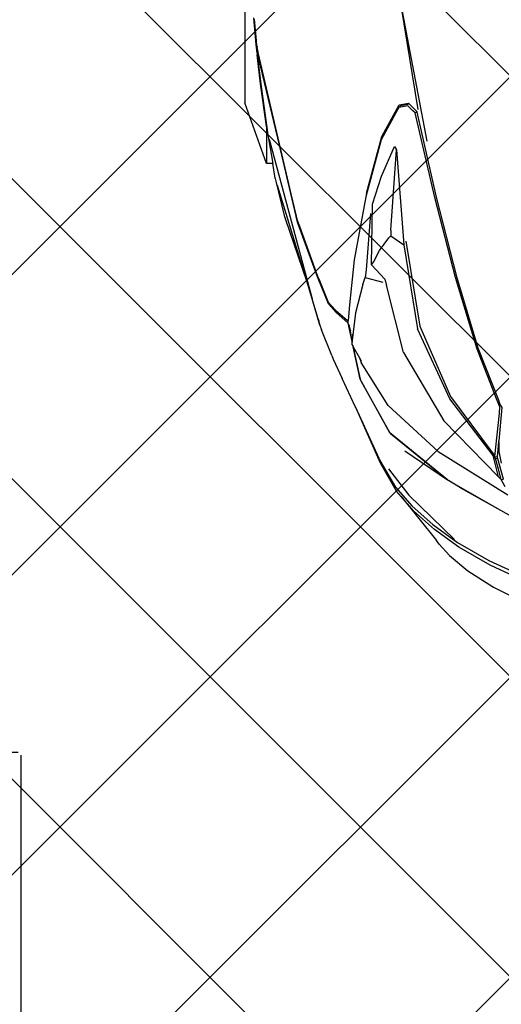
# Model space of a CAD drawing. Units: inches. Extents: x 2167 to 2589, y 1680 to 2489.
# Tile 3 of 38: x 2251.19 to 2262.53, y 1703.49 to 1726.68. Entities that reach past the tile are written whole.
import ezdxf

# ---------------------------------------------------------------- set-up
doc = ezdxf.new("R2010")
doc.units = ezdxf.units.IN
doc.header["$MEASUREMENT"] = 0
doc.layers.get('0').update_dxf_attribs({"color": 250})
for name, color, linetype, lineweight in [('A-ANNO-DIMS', 2, 'Continuous', 18), ('C-PRKG-VEHS', 8, 'Continuous', 13), ('L-PVMT-PATT', 252, 'Continuous', 13)]:
    doc.layers.add(name, color=color, linetype=linetype, lineweight=lineweight)
doc.layers.add('Edges', color=250, linetype='Continuous')
doc.styles.get("Standard").update_dxf_attribs({"font": 'arial.ttf'})
doc.dimstyles.get("Standard").update_dxf_attribs({"dimtxt": 7, "dimasz": 0.18, "dimexe": 0.18, "dimexo": 0.0625, "dimgap": 0.09, "dimtad": 0, "dimtih": 1, "dimtoh": 1, "dimdec": 1, "dimzin": 0, "dimdsep": 46, "dimlunit": 3, "dimtxsty": 'Standard', "dimcen": 0.09, "dimadec": 0, "dimazin": 0, "dimtfac": 1, "dimtdec": 1, "dimtofl": 0, "dimtmove": 0, "dimatfit": 3, "dimfxl": 1, "dimtolj": 1, "dimtzin": 0, "dimarcsym": 0})

# ---------------------------------------------------------------- blocks, each defined once
blk = doc.blocks.new('Nissan Qashqai pl')
at = {"layer": 'Edges'}
for p, q in [((11.47322, 11.2592), (11.46579, 11.24614)), ((11.50736, 11.23616), (11.51652, 11.25601)), ((11.52058, 11.25724), (11.51126, 11.23721)), ((11.52949, 11.24004), (11.53843, 11.2583)), ((11.41698, 11.19425), (11.45295, 11.25195)), ((11.43996, 11.24823), (11.42296, 11.24352)), ((11.44027, 11.24637), (11.43996, 11.24823)), ((11.44624, 11.24948), (11.44027, 11.24637)), ((11.33108, 11.22699), (11.37506, 11.24429)), ((11.37475, 11.24309), (11.33228, 11.22637)), ((11.42033, 11.23975), (11.37334, 11.20375)), ((11.38, 11.24532), (11.37475, 11.24309)), ((11.37506, 11.24429), (11.37524, 11.24436)), ((11.37506, 11.24429), (11.37621, 11.24429)), ((11.37922, 11.24593), (11.37524, 11.24436)), ((11.3763, 11.24436), (11.37524, 11.24436)), ((11.37922, 11.24593), (11.38041, 11.24692)), ((11.37933, 11.24631), (11.37922, 11.24593)), ((11.38533, 11.24487), (11.38, 11.24532)), ((11.38041, 11.24692), (11.40818, 11.24436)), ((11.42115, 11.24117), (11.38533, 11.24487)), ((11.3915, 11.19885), (11.4381, 11.24397)), ((11.41644, 11.24436), (11.40818, 11.24436)), ((11.40898, 11.24429), (11.40818, 11.24436)), ((11.40898, 11.24429), (11.4163, 11.24429)), ((11.4152, 11.24371), (11.40898, 11.24429)), ((11.4163, 11.24429), (11.4152, 11.24371)), ((11.42154, 11.24313), (11.4152, 11.24371)), ((11.41644, 11.24436), (11.4163, 11.24429)), ((11.41686, 11.24458), (11.41644, 11.24436)), ((11.4252, 11.2462), (11.41686, 11.24458)), ((11.41772, 11.23895), (11.41931, 11.23998)), ((11.41915, 11.23969), (11.4194, 11.23996)), ((11.41931, 11.23998), (11.4196, 11.24017)), ((11.4194, 11.23996), (11.41931, 11.23998)), ((11.4194, 11.23996), (11.4196, 11.24017)), ((11.41958, 11.23992), (11.4194, 11.23996)), ((11.4196, 11.24017), (11.42014, 11.24052)), ((11.41984, 11.24006), (11.42014, 11.24052)), ((11.42014, 11.24052), (11.42115, 11.24117)), ((11.42915, 11.24177), (11.42033, 11.23975)), ((11.42287, 11.24164), (11.42033, 11.23975)), ((11.42115, 11.24117), (11.42154, 11.24313)), ((11.42178, 11.24134), (11.42115, 11.24117)), ((11.42296, 11.24352), (11.42154, 11.24313)), ((11.42287, 11.24164), (11.42178, 11.24134)), ((11.42216, 11.24127), (11.42178, 11.24134)), ((11.43154, 11.24397), (11.42287, 11.24164)), ((11.42296, 11.24352), (11.42287, 11.24164)), ((11.42659, 11.2465), (11.4252, 11.2462)), ((11.4381, 11.24397), (11.42915, 11.24177)), ((11.44027, 11.24637), (11.43154, 11.24397)), ((11.4381, 11.24397), (11.44027, 11.24637)), ((11.44114, 11.20281), (11.46562, 11.24583)), ((11.44697, 11.21272), (11.46562, 11.24583)), ((11.46562, 11.24583), (11.46579, 11.24614)), ((11.51576, 11.21859), (11.52949, 11.24004)), ((11.3715, 11.20434), (11.41772, 11.23895)), ((11.49236, 11.21027), (11.50736, 11.23616)), ((11.51126, 11.23721), (11.49628, 11.21137)), ((11.27199, 11.20923), (11.33108, 11.22699)), ((11.33228, 11.22637), (11.27276, 11.20843)), ((11.50327, 11.20341), (11.51576, 11.21859)), ((11.20627, 11.19262), (11.27199, 11.20923)), ((11.27276, 11.20843), (11.20665, 11.19145)), ((11.44697, 11.21272), (11.44114, 11.20281)), ((11.45306, 11.16974), (11.48975, 11.20767)), ((11.47745, 11.18983), (11.49236, 11.21027)), ((11.49628, 11.21137), (11.48154, 11.19102)), ((11.31316, 11.17892), (11.3715, 11.20434)), ((11.37334, 11.20375), (11.31527, 11.17691)), ((11.33497, 11.16556), (11.3915, 11.19885)), ((11.44046, 11.20182), (11.40144, 11.15414)), ((11.40216, 11.15476), (11.44046, 11.20182)), ((11.41633, 11.16662), (11.44046, 11.20182)), ((11.44081, 11.20225), (11.44046, 11.20182)), ((11.4411, 11.20277), (11.44081, 11.20225)), ((11.44114, 11.20281), (11.4411, 11.20277)), ((11.50327, 11.20341), (11.49363, 11.19502)), ((11.20665, 11.19145), (11.14012, 11.17593)), ((11.14803, 11.17913), (11.20627, 11.19262)), ((11.37896, 11.15265), (11.41698, 11.19425)), ((11.45433, 11.16358), (11.49082, 11.19282)), ((11.48154, 11.19102), (11.46617, 11.17358)), ((11.49363, 11.19502), (11.49082, 11.19282)), ((11.03575, 11.16129), (11.1598, 11.18473)), ((11.46237, 11.17248), (11.47745, 11.18983)), ((11.04919, 11.16347), (11.13359, 11.17719)), ((11.12929, 11.17052), (11.13526, 11.17642)), ((11.13658, 11.17502), (11.1347, 11.17313)), ((11.13526, 11.17642), (11.13585, 11.17654)), ((11.13585, 11.17654), (11.14803, 11.17913)), ((11.13585, 11.17654), (11.13658, 11.17502)), ((11.14012, 11.17593), (11.13658, 11.17502)), ((11.24278, 11.16729), (11.31316, 11.17892)), ((11.24587, 11.16563), (11.31527, 11.17691)), ((11.12846, 11.16971), (11.12929, 11.17052)), ((11.12977, 11.16183), (11.12846, 11.16971)), ((11.12929, 11.17052), (11.13057, 11.16299)), ((11.1347, 11.17313), (11.13062, 11.16899)), ((11.13062, 11.16899), (11.13192, 11.16144)), ((11.43143, 11.15309), (11.45306, 11.16974)), ((11.44642, 11.15882), (11.46237, 11.17248)), ((11.46617, 11.17358), (11.45433, 11.16358)), ((11.15597, 11.14759), (11.12977, 11.16183)), ((11.13192, 11.16144), (11.13057, 11.16299)), ((11.13192, 11.16144), (11.13652, 11.15905)), ((11.13652, 11.15905), (11.15893, 11.14704)), ((11.16444, 11.15792), (11.16717, 11.15976)), ((11.18896, 11.14734), (11.16444, 11.15792)), ((11.16717, 11.15976), (11.24587, 11.16563)), ((11.23369, 11.15498), (11.16717, 11.15976)), ((11.23823, 11.15494), (11.24587, 11.16563)), ((11.33497, 11.16556), (11.27913, 11.15147)), ((11.42433, 11.14593), (11.44642, 11.15882)), ((11.44983, 11.15977), (11.42671, 11.14629)), ((11.45433, 11.16358), (11.44983, 11.15977)), ((11.23369, 11.15498), (11.23823, 11.15494)), ((11.23823, 11.15494), (11.2401, 11.15337)), ((11.25046, 11.1455), (11.2401, 11.15337)), ((11.27429, 11.14993), (11.26224, 11.13901)), ((11.27429, 11.14993), (11.27913, 11.15147)), ((11.37896, 11.15265), (11.34336, 11.13032)), ((11.40144, 11.15414), (11.3571, 11.12956)), ((11.35832, 11.12998), (11.40144, 11.15414)), ((11.40216, 11.15476), (11.40144, 11.15414)), ((11.20291, 11.13489), (11.15597, 11.14759)), ((11.15893, 11.14704), (11.20616, 11.13437)), ((11.2121, 11.1399), (11.18896, 11.14734)), ((11.26005, 11.1405), (11.25046, 11.1455)), ((11.27289, 11.13379), (11.27664, 11.14845)), ((11.42671, 11.14629), (11.38067, 11.12595)), ((11.42283, 11.14525), (11.38067, 11.12595)), ((11.42283, 11.14525), (11.42433, 11.14593)), ((11.20291, 11.13489), (11.20295, 11.13488)), ((11.20295, 11.13488), (11.20616, 11.13437)), ((11.20616, 11.13437), (11.25827, 11.12461)), ((11.26224, 11.13901), (11.2121, 11.1399)), ((11.21991, 11.1382), (11.26663, 11.13449)), ((11.26224, 11.13901), (11.26005, 11.1405)), ((11.26663, 11.13449), (11.27289, 11.13379)), ((11.27871, 11.13184), (11.27289, 11.13379)), ((11.27871, 11.13184), (11.30218, 11.1256)), ((11.30218, 11.1256), (11.32517, 11.12286)), ((11.32955, 11.12347), (11.3571, 11.12956)), ((11.3571, 11.12956), (11.33021, 11.12384)), ((11.33021, 11.12384), (11.33938, 11.12898)), ((11.33938, 11.12898), (11.34202, 11.13045)), ((11.33938, 11.12898), (11.34336, 11.13032)), ((11.37962, 11.12547), (11.35656, 11.11477)), ((11.3571, 11.12956), (11.35832, 11.12998)), ((11.38067, 11.12595), (11.37962, 11.12547)), ((11.25827, 11.12461), (11.29558, 11.12077)), ((11.29558, 11.12077), (11.30849, 11.1195)), ((11.30003, 11.10916), (11.30813, 11.11883)), ((11.31027, 11.11923), (11.30178, 11.10961)), ((11.30805, 11.11884), (11.30863, 11.11948)), ((11.30813, 11.11883), (11.30863, 11.11948)), ((11.30849, 11.1195), (11.30863, 11.11948)), ((11.30863, 11.11948), (11.31033, 11.1193)), ((11.31033, 11.1193), (11.31027, 11.11923)), ((11.31033, 11.1193), (11.31061, 11.11927)), ((11.31061, 11.11927), (11.314, 11.12039)), ((11.31704, 11.12142), (11.31186, 11.12058)), ((11.31323, 11.11986), (11.32588, 11.12266)), ((11.32423, 11.12258), (11.314, 11.12039)), ((11.314, 11.12039), (11.31704, 11.12142)), ((11.32423, 11.12258), (11.31704, 11.12142)), ((11.31982, 11.1231), (11.32517, 11.12286)), ((11.32423, 11.12258), (11.32588, 11.12266)), ((11.32517, 11.12286), (11.32831, 11.12278)), ((11.32588, 11.12266), (11.32831, 11.12278)), ((11.32831, 11.12278), (11.32955, 11.12347)), ((11.32955, 11.12347), (11.33021, 11.12384)), ((11.29339, 11.10313), (11.30003, 11.10916)), ((11.30178, 11.10961), (11.29459, 11.10327)), ((11.34052, 11.10725), (11.35656, 11.11477)), ((11.29459, 11.10327), (11.27358, 11.0947)), ((11.27407, 11.09522), (11.29339, 11.10313)), ((11.33757, 11.10603), (11.31612, 11.09747)), ((11.33757, 11.10603), (11.34052, 11.10725)), ((11.2732, 11.09452), (11.22772, 11.07792)), ((11.23038, 11.07923), (11.27187, 11.09432)), ((11.27187, 11.09432), (11.27407, 11.09522)), ((11.27358, 11.0947), (11.2732, 11.09452)), ((11.27358, 11.0947), (11.27407, 11.09522)), ((11.27568, 11.08503), (11.31244, 11.09628)), ((11.31244, 11.09628), (11.29065, 11.08989)), ((11.30801, 11.09508), (11.30877, 11.09528)), ((11.31244, 11.09628), (11.31612, 11.09747)), ((11.15816, 11.05423), (11.29065, 11.08989)), ((11.19633, 11.06072), (11.27568, 11.08503)), ((11.22475, 11.06772), (11.27568, 11.08503)), ((11.22216, 11.0766), (11.08821, 11.045)), ((11.09177, 11.04531), (11.22216, 11.0766)), ((11.21998, 11.07614), (11.22216, 11.0766)), ((11.2222, 11.07656), (11.22216, 11.0766)), ((11.22715, 11.07771), (11.2222, 11.07656)), ((11.22238, 11.07665), (11.2222, 11.07656)), ((11.22238, 11.07665), (11.22532, 11.07737)), ((11.22532, 11.07737), (11.23038, 11.07923)), ((11.22731, 11.07783), (11.22706, 11.07777)), ((11.22962, 11.07837), (11.22715, 11.07771)), ((11.22772, 11.07792), (11.22715, 11.07771)), ((11.22962, 11.07837), (11.22772, 11.07792)), ((11.08649, 11.04496), (11.21998, 11.07614)), ((11.19297, 11.05964), (11.22148, 11.06662)), ((11.22148, 11.06662), (11.22475, 11.06772)), ((11.14751, 11.05208), (11.11234, 11.04716)), ((11.11474, 11.04762), (11.15472, 11.05317)), ((11.17828, 11.05208), (11.12828, 11.03408)), ((11.15248, 11.05278), (11.14751, 11.05208)), ((11.14751, 11.05208), (11.17828, 11.05208)), ((11.15472, 11.05317), (11.15248, 11.05278)), ((11.15472, 11.05317), (11.17828, 11.05716)), ((11.19065, 11.05923), (11.17828, 11.05716)), ((11.17828, 11.05716), (11.17828, 11.05208)), ((11.19089, 11.05929), (11.19065, 11.05923)), ((11.19089, 11.05929), (11.19297, 11.05964)), ((11.07681, 11.04337), (11.08106, 11.04371)), ((11.08696, 11.04422), (11.07977, 11.04339)), ((11.08106, 11.04371), (11.08273, 11.0441)), ((11.08114, 11.04436), (11.08208, 11.0442)), ((11.08273, 11.0441), (11.08562, 11.04476)), ((11.08273, 11.0441), (11.08365, 11.04395)), ((11.08821, 11.045), (11.08365, 11.04395)), ((11.08365, 11.04395), (11.08696, 11.04422)), ((11.08562, 11.04476), (11.08649, 11.04496)), ((11.08649, 11.04496), (11.08796, 11.04514)), ((11.08696, 11.04422), (11.08721, 11.04424)), ((11.08728, 11.04426), (11.08721, 11.04424)), ((11.08728, 11.04426), (11.08834, 11.04438)), ((11.08834, 11.04438), (11.11474, 11.04762)), ((11.11234, 11.04716), (11.08834, 11.04438)), ((11.07977, 11.04339), (11.05762, 11.04159)), ((11.05899, 11.04188), (11.07681, 11.04337)), ((10.95773, 11.03408), (11.12828, 11.03408))]:
    blk.add_line(p, q, dxfattribs=at)
blk = doc.blocks.new('car')
blk.add_blockref('Nissan Qashqai pl', (-9.74328, -11.91512))
blk = doc.blocks.new('carr')
blk.add_blockref('car', (0.51244, -0.00696))
blk = doc.blocks.new('*D45')
at = {"layer": 'A-ANNO-DIMS', "color": 0, "lineweight": -2, "transparency": 16777216}
for p, q in [((2251.156, 1833.955), (2232.359, 1833.955)), ((2232.539, 1833.775), (2232.539, 1775.399)), ((2232.539, 1709.605), (2232.539, 1767.981)), ((2251.156, 1709.425), (2232.359, 1709.425))]:
    blk.add_line(p, q, dxfattribs=at)
at = {"layer": 'A-ANNO-DIMS', "color": 0, "transparency": 16777216}
for points in [[(2232.509, 1833.775), (2232.569, 1833.775), (2232.539, 1833.955)], [(2232.509, 1709.605), (2232.569, 1709.605), (2232.539, 1709.425)]]:
    blk.add_solid(points, dxfattribs=at)
at = {"layer": 'Defpoints', "color": 0, "transparency": 16777216}
for p in [(2251.218, 1833.955), (2232.539, 1709.425), (2251.218, 1709.425)]:
    blk.add_point(p, dxfattribs=at)
at = {"layer": 'A-ANNO-DIMS', "color": 0, "transparency": 16777216, "insert": (2232.539, 1771.69), "char_height": 7, "attachment_point": 5}
blk.add_mtext('\\A1;CAR 10\'-4 1/2" TYP.', dxfattribs=at)
blk = doc.blocks.new('*D46')
at = {"layer": 'A-ANNO-DIMS', "color": 0, "lineweight": -2, "transparency": 16777216}
for p, q in [((2251.218, 1709.362), (2251.218, 1690.565)), ((2312.254, 1709.362), (2312.254, 1690.565)), ((2251.398, 1690.745), (2260.312, 1690.745)), ((2312.074, 1690.745), (2303.16, 1690.745))]:
    blk.add_line(p, q, dxfattribs=at)
at = {"layer": 'A-ANNO-DIMS', "color": 0, "transparency": 16777216}
for points in [[(2251.398, 1690.775), (2251.398, 1690.715), (2251.218, 1690.745)], [(2312.074, 1690.775), (2312.074, 1690.715), (2312.254, 1690.745)]]:
    blk.add_solid(points, dxfattribs=at)
at = {"layer": 'Defpoints', "color": 0, "transparency": 16777216}
for p in [(2251.218, 1709.425), (2312.254, 1709.425), (2312.254, 1690.745)]:
    blk.add_point(p, dxfattribs=at)
at = {"layer": 'A-ANNO-DIMS', "color": 0, "transparency": 16777216, "insert": (2281.736, 1690.745), "char_height": 7, "attachment_point": 5}
blk.add_mtext('\\A1;5\'-1" TYP.', dxfattribs=at)

msp = doc.modelspace()

# ---------------------------------------------------------------- hatches: boundary and pattern name
at = {"layer": 'L-PVMT-PATT'}
h = msp.add_hatch(dxfattribs=at)
h.set_pattern_fill('ANSI37', color=256, scale=40)
h.paths.add_polyline_path([(2417.548, 1783.695), (2417.548, 1846.042), (2239.361, 1846.042), (2239.361, 1687.695), (2369.843, 1687.695), (2369.843, 1696.695), (2375.607, 1696.695), (2416.107, 1696.695), (2417.548, 1696.695)])

# ---------------------------------------------------------------- block references
at = {"layer": 'C-PRKG-VEHS', "xscale": 28.42784210623918, "yscale": 28.42784210623918, "zscale": 28.42784210623918, "rotation": 270}
msp.add_blockref('carr', (2281.736, 1778.659), dxfattribs=at)

# ---------------------------------------------------------------- dimensions: what is measured, and where the dimension line sits
at = {"layer": 'A-ANNO-DIMS'}
dim = msp.add_linear_dim(base=(2232.539, 1709.425), p1=(2251.218, 1833.955), p2=(2251.218, 1709.425), angle=270, text='CAR <> TYP.', dimstyle='Standard', override={"dimdec": 1, "dimlfac": 1, "dimrnd": 0, "dimzin": 1, "dimdsep": 46, "dimlunit": 4, "dimfrac": 2}, dxfattribs=at)
dim.commit()
dim.dimension.update_dxf_attribs({"geometry": '*D45', "text_midpoint": (2232.539, 1771.69)})
dim = msp.add_linear_dim(base=(2312.254, 1690.745), p1=(2251.218, 1709.425), p2=(2312.254, 1709.425), text='<> TYP.', dimstyle='Standard', override={"dimdec": 1, "dimlfac": 1, "dimrnd": 0, "dimzin": 1, "dimdsep": 46, "dimlunit": 4, "dimfrac": 2}, dxfattribs=at)
dim.commit()
dim.dimension.update_dxf_attribs({"geometry": '*D46', "text_midpoint": (2281.736, 1690.745)})

doc.saveas('drawing.dxf')
